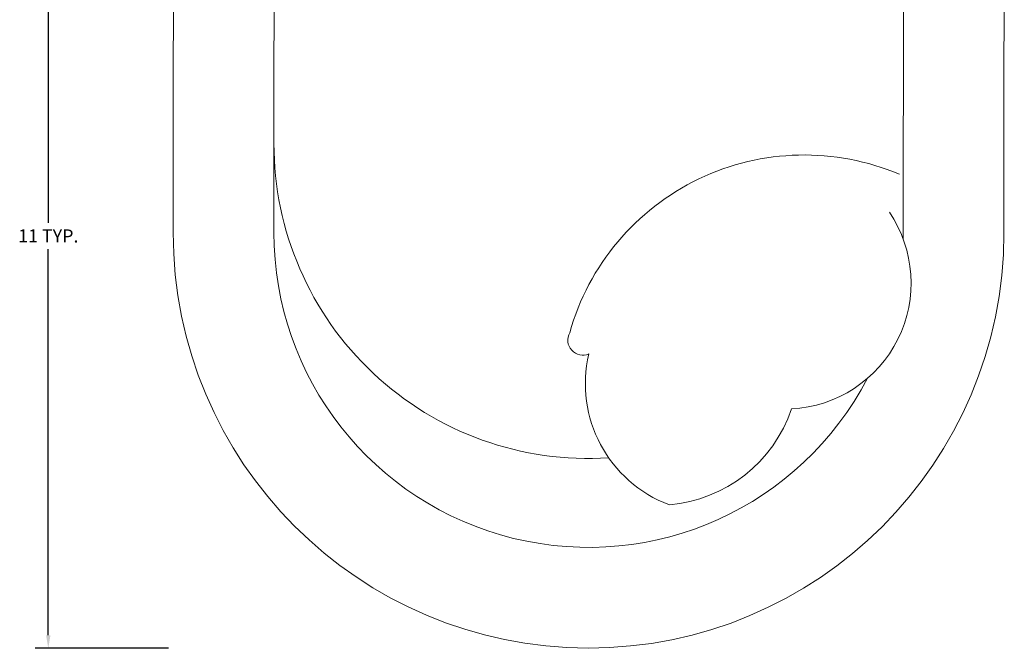
# Model space of a CAD drawing. Units: inches. Extents: x 2168 to 3056, y 1130 to 2629.
# Tile 9 of 42: x 2669.42 to 2682.96, y 1970.61 to 1979.25. Entities that reach past the tile are written whole.
import ezdxf

# ---------------------------------------------------------------- set-up
doc = ezdxf.new("R2010")
doc.units = ezdxf.units.IN
doc.layers.add('A-ANNO-DIMS', color=2, linetype='Continuous', lineweight=18)
doc.layers.add('A-FURN', color=8, linetype='Continuous', lineweight=13)
doc.styles.get("Standard").update_dxf_attribs({"font": 'arial.ttf'})
doc.dimstyles.get("Standard").update_dxf_attribs({"dimtxt": 0.18, "dimasz": 0.18, "dimexe": 0.18, "dimexo": 0.0625, "dimgap": 0.09, "dimtad": 0, "dimtih": 1, "dimtoh": 1, "dimdec": 4, "dimzin": 0, "dimdsep": 46, "dimtxsty": 'Standard', "dimcen": 0.09, "dimadec": 0, "dimazin": 0, "dimtfac": 1, "dimtdec": 4, "dimtofl": 0, "dimtmove": 0, "dimatfit": 3, "dimfxl": 1, "dimtolj": 1, "dimtzin": 0, "dimarcsym": 0})

# ---------------------------------------------------------------- blocks, each defined once
blk = doc.blocks.new('CHAIR-LOUNGE')
blk.add_line((10.035, 5.706), (10.04, 10.985))
at = {"ltscale": 0.03}
blk.add_lwpolyline([(10.04, 10.985, -0.369229), (11.424, 10.983), (11.419, 5.705, -1), (0, 5.715), (0.005, 10.994, -0.369229), (1.389, 10.993)], format="xyb", close=True, dxfattribs=at)
blk.add_lwpolyline([(9.546, 3.712, -0.785087), (1.384, 5.714), (1.389, 10.993)], format="xyb")
for centre, radius, start, end in [((5.711, 6.932), 4.326, 179.9461, 273.658), ((8.675, 3.429), 3.35, 67.0143, 164.2857), ((8.409, 5.02), 1.734, 272.9922, 34.1401), ((5.709, 5.71), 4.326, 358.8536, 359.9461), ((5.631, 4.234), 0.207, 150.6238, 293.7423), ((7.444, 3.634), 1.778, 166.6403, 249.4695), ((6.65, 3.913), 1.951, 274.9999, 341.3534)]:
    blk.add_arc(centre, radius, start, end)
blk = doc.blocks.new('*D17')
at = {"layer": 'A-ANNO-DIMS', "color": 0, "lineweight": -2, "transparency": 16777216}
for p, q in [((2671.469, 1981.947), (2669.638, 1981.947)), ((2669.818, 1981.767), (2669.818, 1976.459)), ((2669.818, 1970.79), (2669.818, 1976.098)), ((2671.469, 1970.61), (2669.638, 1970.61))]:
    blk.add_line(p, q, dxfattribs=at)
at = {"layer": 'A-ANNO-DIMS', "color": 0, "transparency": 16777216}
for points in [[(2669.788, 1981.767), (2669.848, 1981.767), (2669.818, 1981.947)], [(2669.788, 1970.79), (2669.848, 1970.79), (2669.818, 1970.61)]]:
    blk.add_solid(points, dxfattribs=at)
at = {"layer": 'Defpoints', "color": 0, "transparency": 16777216}
for p in [(2669.818, 1981.947), (2671.532, 1981.947), (2671.532, 1970.61)]:
    blk.add_point(p, dxfattribs=at)
at = {"layer": 'A-ANNO-DIMS', "color": 0, "transparency": 16777216, "insert": (2669.818, 1976.278), "char_height": 0.18, "attachment_point": 5}
blk.add_mtext('\\A1;11 TYP.', dxfattribs=at)

msp = doc.modelspace()

# ---------------------------------------------------------------- block references
at = {"layer": 'A-FURN'}
msp.add_blockref('CHAIR-LOUNGE', (2671.535, 1970.612), dxfattribs=at)

# ---------------------------------------------------------------- dimensions: what is measured, and where the dimension line sits
at = {"layer": 'A-ANNO-DIMS'}
dim = msp.add_linear_dim(base=(2669.818, 1981.947), p1=(2671.532, 1970.61), p2=(2671.532, 1981.947), angle=90, text='<> TYP.', dimstyle='Standard', override={"dimdec": 0, "dimlfac": 1, "dimrnd": 0, "dimzin": 0, "dimdsep": 46, "dimlunit": 2}, dxfattribs=at)
dim.commit()
dim.dimension.update_dxf_attribs({"geometry": '*D17', "text_midpoint": (2669.818, 1976.278)})

doc.saveas('drawing.dxf')
